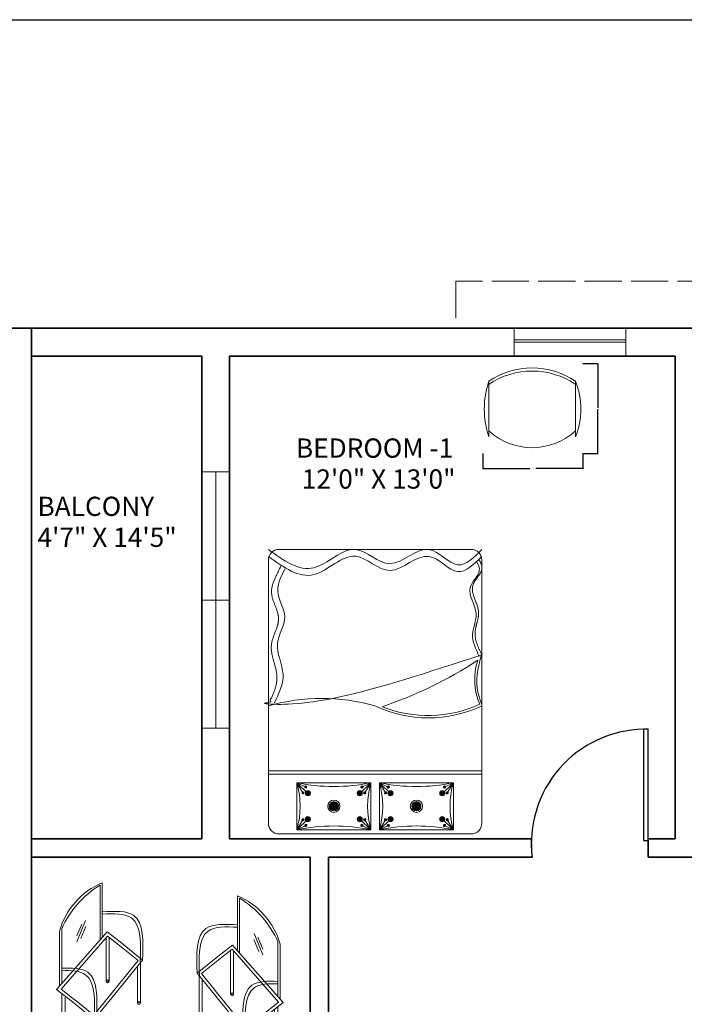
# Model space of a CAD drawing. Units: inches. Extents: x -61 to 1599, y -1316 to 257.
# Tile 201 of 204: x 998 to 1213, y -61 to 257. Entities that reach past the tile are written whole.
import ezdxf

# ---------------------------------------------------------------- set-up
doc = ezdxf.new("R2010")
doc.units = ezdxf.units.IN
doc.header["$MEASUREMENT"] = 0
doc.linetypes.add('ACAD_ISO02W100', pattern=[15, 12, -3])
for name, color, linetype, lineweight in [('A-ANNO-DIMS', 2, 'Continuous', 18), ('A-AREA-IDEN', 1, 'Continuous', 18), ('A-FLOR-OVHD', 203, 'ACAD_ISO02W100', 13), ('A-WALL-JAMB', 4, 'ACAD_ISO02W100', 25), ('DOORS', 2, 'Continuous', 25), ('FURNITURE', 83, 'Continuous', 18), ('WALLS', 4, 'Continuous', 35), ('WINDOWS', 220, 'Continuous', 18)]:
    doc.layers.add(name, color=color, linetype=linetype, lineweight=lineweight)
doc.layers.add('LT', color=8, linetype='Continuous')
doc.styles.get("Standard").update_dxf_attribs({"font": 'arial.ttf'})
doc.dimstyles.get("Standard").update_dxf_attribs({"dimtxt": 0.18, "dimasz": 0.18, "dimexe": 0.18, "dimexo": 0.0625, "dimgap": 0.09, "dimtad": 0, "dimtih": 1, "dimtoh": 1, "dimdec": 0, "dimzin": 0, "dimdsep": 46, "dimlunit": 3, "dimtxsty": 'Standard', "dimcen": 0.09, "dimadec": 0, "dimazin": 0, "dimtfac": 1, "dimtdec": 0, "dimtofl": 0, "dimtmove": 0, "dimatfit": 3, "dimfxl": 1, "dimtolj": 1, "dimtzin": 0, "dimarcsym": 0})

# ---------------------------------------------------------------- blocks, each defined once
blk = doc.blocks.new('DOOR-SWING-36')
blk.add_line((0, 0), (0, -5.4))
blk.add_lwpolyline([(0, 0), (0, 36), (-1.57, 36), (-1.57, 0)], close=True)
blk.add_arc((-0.74, -1.08), 37.09, 91.2913, 186.6905)
blk = doc.blocks.new('WIN-36IN')
for p, q in [((0, 4.5), (0, 9)), ((0, 9), (0, 0)), ((36, 9), (36, 0)), ((0, 5.26), (36, 5.26)), ((0, 4.5), (36, 4.5)), ((0, 4.5), (36, 4.5))]:
    blk.add_line(p, q)
blk = doc.blocks.new('WIN-83IN')
for p, q in [((0, 82.94), (9, 82.94)), ((0, 0), (9, 0))]:
    blk.add_line(p, q)
for points in [[(9, 82.94), (4.5, 82.94), (4.5, 41.47), (9, 41.47)], [(4.5, 41.47), (0, 41.47), (0, 0), (4.5, 0)]]:
    blk.add_lwpolyline(points, close=True)
blk = doc.blocks.new('BEDROOM-CHAIR')
for p, q in [((1.45, 3.47), (1.45, 21.47)), ((29.49, 3.47), (29.49, 21.47))]:
    blk.add_line(p, q)
for centre, radius, start, end in [((15.47, 0.83), 24.95, 55.8098, 124.1902), ((15.47, -0.17), 24.95, 55.8098, 124.1902), ((28.58, 12.47), 28.58, 161.6455, 198.3545), ((7.26, 12.47), 23.99, 337.9646, 22.0354), ((15.47, 20.69), 20.68, 227.332, 312.668)]:
    blk.add_arc(centre, radius, start, end)
blk = doc.blocks.new('LOUNGE-CHAIR')
for p, q in [((14.04, 40.33), (14.04, 58.08)), ((14.76, 41.14), (14.76, 58.89)), ((6.52, 39.78), (9.29, 46.65)), ((6.58, 41.68), (8.18, 45.54)), ((7.84, 40.87), (9.45, 44.74)), ((0, 24.35), (16.38, 42.98)), ((0.97, 25.45), (0.97, 43.2)), ((0.97, 25.45), (0.97, 43.2)), ((1.45, 24.49), (16.5, 41.61)), ((1.64, 26.22), (1.64, 43.97)), ((16.38, 42.98), (20.51, 39.74)), ((16.5, 41.61), (19.89, 38.96)), ((16.97, 42.52), (16.97, 42.52)), ((15.97, 27.05), (15.97, 41.01)), ((16.97, 27.05), (16.97, 41.25)), ((19.88, 38.97), (26.35, 33.72)), ((20.51, 39.74), (27.76, 33.87)), ((12.02, 16.03), (26.35, 33.72)), ((12.16, 14.63), (27.76, 33.87)), ((27.1, 20.02), (27.1, 33.05)), ((26.1, 20.02), (26.1, 31.82)), ((16.97, 27.05), (15.97, 27.05)), ((0, 24.35), (5.1, 20.35)), ((0.75, 23.69), (0.79, 23.74)), ((1.45, 24.49), (5.72, 21.14)), ((1.73, 7.53), (1.73, 23)), ((2.73, 7.53), (2.73, 22.21)), ((5.1, 20.35), (12.16, 14.63)), ((5.73, 21.13), (12.02, 16.03)), ((27.1, 20.02), (26.1, 20.02)), ((11.85, 0.5), (11.85, 14.88)), ((12.85, 0.5), (12.85, 15.48)), ((2.73, 7.53), (1.73, 7.53)), ((12.85, 0.5), (11.85, 0.5))]:
    blk.add_line(p, q)
for centre in [(16.47, 27.05), (26.6, 20.02), (2.23, 7.53), (12.35, 0.5)]:
    blk.add_circle(centre, 0.5)
for centre, radius, start, end in [((23.93, 36.92), 23.8, 112.6586, 164.6996), ((30.25, 31.33), 31.28, 121.203, 156.1552)]:
    blk.add_arc(centre, radius, start, end)
for points, knots in [([(14.76, 49.49), (18.73, 49.7), (28.38, 50.23), (27.99, 39.93), (27.76, 33.87)], [0, 0, 0, 0, 10.281855, 24.983674, 24.983674, 24.983674, 24.983674]), ([(14.76, 48.72), (18.48, 48.91), (27.65, 49.16), (27.27, 39.12), (27.05, 33.06), (27.04, 33.03), (27.04, 33.01), (27.04, 32.98)], [0.614676, 0.614676, 0.614676, 0.614676, 10.281855, 24.983674, 24.983674, 24.983674, 25.041855, 25.041855, 25.041855, 25.041855]), ([(1.64, 31.22), (4.99, 31.37), (13.47, 31.24), (13.11, 21.57), (12.88, 15.51)], [1.527723, 1.527723, 1.527723, 1.527723, 10.281855, 24.983674, 24.983674, 24.983674, 24.983674]), ([(1.64, 30.44), (4.72, 30.55), (12.75, 30.17), (12.39, 20.76), (12.17, 14.7), (12.16, 14.67), (12.16, 14.65), (12.16, 14.63)], [2.150702, 2.150702, 2.150702, 2.150702, 10.281855, 24.983674, 24.983674, 24.983674, 25.041855, 25.041855, 25.041855, 25.041855])]:
    blk.add_open_spline(points, degree=3, knots=knots)
blk = doc.blocks.new('*U15')
at = {"layer": 'LT'}
blk.add_line((0, 0.18), (0, -0.18), dxfattribs=at)
for centre, start, end in [((0.51, 0), 160.9983, 199.0017), ((-0.51, 0), 340.9983, 19.0017)]:
    blk.add_arc(centre, 0.539, start, end, dxfattribs=at)
blk = doc.blocks.new('*U16')
at = {"layer": 'LT', "transparency": 16777216}
for p, rotation in [((-66.65, -18.83), 96), ((-66.64, -18.76), 72), ((-66.63, -18.9), 120), ((-66.61, -18.69), 48.00000000000001), ((-66.58, -18.95), 144), ((-66.55, -18.65), 24), ((-66.51, -18.98), 168.0000000000001), ((-66.4, -18.65), 336.0000000000001), ((-66.37, -18.95), 216), ((-66.44, -18.98), 192), ((-66.34, -18.69), 312), ((-66.32, -18.9), 240), ((-66.31, -18.76), 288.0000000000001), ((-66.3, -18.83), 264)]:
    blk.add_blockref('*U15', p, dxfattribs=dict(at, rotation=rotation))
blk.add_blockref('*U15', (-66.48, -18.63), dxfattribs=at)
blk = doc.blocks.new('*U45')
at = {"layer": 'LT'}
blk.add_line((0, 0.18), (0, -0.18), dxfattribs=at)
for centre, start, end in [((0.51, 0), 160.9983, 199.0017), ((-0.51, 0), 340.9983, 19.0017)]:
    blk.add_arc(centre, 0.539, start, end, dxfattribs=at)
blk = doc.blocks.new('*U46')
at = {"layer": 'LT', "transparency": 16777216}
for p, rotation in [((-66.65, -18.83), 96), ((-66.64, -18.76), 72), ((-66.63, -18.9), 120), ((-66.61, -18.69), 48.00000000000001), ((-66.58, -18.95), 144), ((-66.55, -18.65), 24), ((-66.51, -18.98), 168.0000000000001), ((-66.4, -18.65), 336.0000000000001), ((-66.37, -18.95), 216), ((-66.44, -18.98), 192), ((-66.34, -18.69), 312), ((-66.32, -18.9), 240), ((-66.31, -18.76), 288.0000000000001), ((-66.3, -18.83), 264)]:
    blk.add_blockref('*U45', p, dxfattribs=dict(at, rotation=rotation))
blk.add_blockref('*U45', (-66.48, -18.63), dxfattribs=at)
blk = doc.blocks.new('*U9')
at = {"layer": 'LT'}
blk.add_line((0, 0.18), (0, -0.18), dxfattribs=at)
for centre, start, end in [((0.51, 0), 160.9983, 199.0017), ((-0.51, 0), 340.9983, 19.0017)]:
    blk.add_arc(centre, 0.539, start, end, dxfattribs=at)
blk = doc.blocks.new('*U10')
at = {"layer": 'LT', "transparency": 16777216}
for p, rotation in [((-66.65, -18.83), 96), ((-66.64, -18.76), 72), ((-66.63, -18.9), 120), ((-66.61, -18.69), 48.00000000000001), ((-66.58, -18.95), 144), ((-66.55, -18.65), 24), ((-66.51, -18.98), 168.0000000000001), ((-66.4, -18.65), 336.0000000000001), ((-66.37, -18.95), 216), ((-66.44, -18.98), 192), ((-66.34, -18.69), 312), ((-66.32, -18.9), 240), ((-66.31, -18.76), 288.0000000000001), ((-66.3, -18.83), 264)]:
    blk.add_blockref('*U9', p, dxfattribs=dict(at, rotation=rotation))
blk.add_blockref('*U9', (-66.48, -18.63), dxfattribs=at)
blk = doc.blocks.new('*U39')
at = {"layer": 'LT'}
blk.add_line((0, 0.18), (0, -0.18), dxfattribs=at)
for centre, start, end in [((0.51, 0), 160.9983, 199.0017), ((-0.51, 0), 340.9983, 19.0017)]:
    blk.add_arc(centre, 0.539, start, end, dxfattribs=at)
blk = doc.blocks.new('*U40')
at = {"layer": 'LT', "transparency": 16777216}
for p, rotation in [((-66.65, -18.83), 96), ((-66.64, -18.76), 72), ((-66.63, -18.9), 120), ((-66.61, -18.69), 48.00000000000001), ((-66.58, -18.95), 144), ((-66.55, -18.65), 24), ((-66.51, -18.98), 168.0000000000001), ((-66.4, -18.65), 336.0000000000001), ((-66.37, -18.95), 216), ((-66.44, -18.98), 192), ((-66.34, -18.69), 312), ((-66.32, -18.9), 240), ((-66.31, -18.76), 288.0000000000001), ((-66.3, -18.83), 264)]:
    blk.add_blockref('*U39', p, dxfattribs=dict(at, rotation=rotation))
blk.add_blockref('*U39', (-66.48, -18.63), dxfattribs=at)
blk = doc.blocks.new('*U17')
at = {"layer": 'LT'}
blk.add_line((0, 0.41), (0, -0.41), dxfattribs=at)
for centre, start, end in [((1.2, 0), 160.9983, 199.0017), ((-1.2, 0), 340.9983, 19.0017)]:
    blk.add_arc(centre, 1.27, start, end, dxfattribs=at)
blk = doc.blocks.new('*U18')
at = {"layer": 'LT', "transparency": 16777216}
for p, rotation in [((-156.74, -44.28), 96), ((-156.73, -44.11), 72), ((-156.69, -44.44), 120), ((-156.64, -43.96), 48.00000000000001), ((-156.58, -44.57), 144), ((-156.5, -43.86), 24), ((-156.42, -44.64), 168), ((-156.17, -43.86), 336.0000000000001), ((-156.25, -44.64), 192), ((-156.09, -44.57), 216), ((-156.03, -43.96), 312), ((-155.98, -44.44), 240), ((-155.94, -44.11), 288.0000000000001), ((-155.92, -44.28), 264)]:
    blk.add_blockref('*U17', p, dxfattribs=dict(at, rotation=rotation))
blk.add_blockref('*U17', (-156.33, -43.82), dxfattribs=at)
blk = doc.blocks.new('*U33')
at = {"layer": 'LT'}
blk.add_line((0, 0.41), (0, -0.41), dxfattribs=at)
for centre, start, end in [((1.2, 0), 160.9983, 199.0017), ((-1.2, 0), 340.9983, 19.0017)]:
    blk.add_arc(centre, 1.27, start, end, dxfattribs=at)
blk = doc.blocks.new('*U34')
at = {"layer": 'LT', "transparency": 16777216}
for p, rotation in [((-156.74, -44.28), 96), ((-156.73, -44.11), 72), ((-156.69, -44.44), 120), ((-156.64, -43.96), 48.00000000000001), ((-156.58, -44.57), 144), ((-156.5, -43.86), 24), ((-156.42, -44.64), 168), ((-156.17, -43.86), 336.0000000000001), ((-156.25, -44.64), 192), ((-156.09, -44.57), 216), ((-156.03, -43.96), 312), ((-155.98, -44.44), 240), ((-155.94, -44.11), 288.0000000000001), ((-155.92, -44.28), 264)]:
    blk.add_blockref('*U33', p, dxfattribs=dict(at, rotation=rotation))
blk.add_blockref('*U33', (-156.33, -43.82), dxfattribs=at)
blk = doc.blocks.new('*U11')
at = {"layer": 'LT'}
blk.add_line((0, 0.74), (0, -0.74), dxfattribs=at)
for centre, start, end in [((2.15, 0), 160.9983, 199.0017), ((-2.15, 0), 340.9983, 19.0017)]:
    blk.add_arc(centre, 2.27, start, end, dxfattribs=at)
blk = doc.blocks.new('*U12')
at = {"layer": 'LT', "transparency": 16777216}
for p, rotation in [((-280.98, -79.37), 96), ((-280.94, -79.07), 72), ((-280.88, -79.67), 120), ((-280.79, -78.8), 48.00000000000001), ((-280.68, -79.89), 144), ((-280.54, -78.62), 23.99999999999999), ((-280.4, -80.02), 168), ((-280.09, -80.02), 191.9999999999999), ((-279.94, -78.62), 336.0000000000001), ((-279.81, -79.89), 216), ((-279.69, -78.8), 312), ((-279.6, -79.67), 240), ((-279.54, -79.07), 288.0000000000001), ((-279.51, -79.37), 264)]:
    blk.add_blockref('*U11', p, dxfattribs=dict(at, rotation=rotation))
blk.add_blockref('*U11', (-280.24, -78.56), dxfattribs=at)
blk = doc.blocks.new('*U28')
at = {"layer": 'LT'}
blk.add_line((0, 0.41), (0, -0.41), dxfattribs=at)
for centre, start, end in [((1.2, 0), 160.9983, 199.0017), ((-1.2, 0), 340.9983, 19.0017)]:
    blk.add_arc(centre, 1.27, start, end, dxfattribs=at)
blk = doc.blocks.new('*U44')
at = {"layer": 'LT', "transparency": 16777216}
for p, rotation in [((-156.74, -44.28), 96), ((-156.73, -44.11), 72), ((-156.69, -44.44), 120), ((-156.64, -43.96), 48.00000000000001), ((-156.58, -44.57), 144), ((-156.5, -43.86), 24), ((-156.42, -44.64), 168), ((-156.17, -43.86), 336.0000000000001), ((-156.25, -44.64), 192), ((-156.09, -44.57), 216), ((-156.03, -43.96), 312), ((-155.98, -44.44), 240), ((-155.94, -44.11), 288.0000000000001), ((-155.92, -44.28), 264)]:
    blk.add_blockref('*U28', p, dxfattribs=dict(at, rotation=rotation))
blk.add_blockref('*U28', (-156.33, -43.82), dxfattribs=at)
blk = doc.blocks.new('*U13')
at = {"layer": 'LT'}
blk.add_line((0, 0.41), (0, -0.41), dxfattribs=at)
for centre, start, end in [((1.2, 0), 160.9983, 199.0017), ((-1.2, 0), 340.9983, 19.0017)]:
    blk.add_arc(centre, 1.27, start, end, dxfattribs=at)
blk = doc.blocks.new('*U14')
at = {"layer": 'LT', "transparency": 16777216}
for p, rotation in [((-156.74, -44.28), 96), ((-156.73, -44.11), 72), ((-156.69, -44.44), 120), ((-156.64, -43.96), 48.00000000000001), ((-156.58, -44.57), 144), ((-156.5, -43.86), 24), ((-156.42, -44.64), 168), ((-156.17, -43.86), 336.0000000000001), ((-156.25, -44.64), 192), ((-156.09, -44.57), 216), ((-156.03, -43.96), 312), ((-155.98, -44.44), 240), ((-155.94, -44.11), 288.0000000000001), ((-155.92, -44.28), 264)]:
    blk.add_blockref('*U13', p, dxfattribs=dict(at, rotation=rotation))
blk.add_blockref('*U13', (-156.33, -43.82), dxfattribs=at)
blk = doc.blocks.new('*U19')
at = {"layer": 'LT'}
blk.add_line((0, 0.18), (0, -0.18), dxfattribs=at)
for centre, start, end in [((0.51, 0), 160.9983, 199.0017), ((-0.51, 0), 340.9983, 19.0017)]:
    blk.add_arc(centre, 0.539, start, end, dxfattribs=at)
blk = doc.blocks.new('*U6')
at = {"layer": 'LT', "transparency": 16777216}
for p, rotation in [((-66.65, -18.83), 96), ((-66.64, -18.76), 72), ((-66.63, -18.9), 120), ((-66.61, -18.69), 48.00000000000001), ((-66.58, -18.95), 144), ((-66.55, -18.65), 24), ((-66.51, -18.98), 168.0000000000001), ((-66.4, -18.65), 336.0000000000001), ((-66.37, -18.95), 216), ((-66.44, -18.98), 192), ((-66.34, -18.69), 312), ((-66.32, -18.9), 240), ((-66.31, -18.76), 288.0000000000001), ((-66.3, -18.83), 264)]:
    blk.add_blockref('*U19', p, dxfattribs=dict(at, rotation=rotation))
blk.add_blockref('*U19', (-66.48, -18.63), dxfattribs=at)
blk = doc.blocks.new('*U35')
at = {"layer": 'LT'}
blk.add_line((0, 0.18), (0, -0.18), dxfattribs=at)
for centre, start, end in [((0.51, 0), 160.9983, 199.0017), ((-0.51, 0), 340.9983, 19.0017)]:
    blk.add_arc(centre, 0.539, start, end, dxfattribs=at)
blk = doc.blocks.new('*U36')
at = {"layer": 'LT', "transparency": 16777216}
for p, rotation in [((-66.65, -18.83), 96), ((-66.64, -18.76), 72), ((-66.63, -18.9), 120), ((-66.61, -18.69), 48.00000000000001), ((-66.58, -18.95), 144), ((-66.55, -18.65), 24), ((-66.51, -18.98), 168.0000000000001), ((-66.4, -18.65), 336.0000000000001), ((-66.37, -18.95), 216), ((-66.44, -18.98), 192), ((-66.34, -18.69), 312), ((-66.32, -18.9), 240), ((-66.31, -18.76), 288.0000000000001), ((-66.3, -18.83), 264)]:
    blk.add_blockref('*U35', p, dxfattribs=dict(at, rotation=rotation))
blk.add_blockref('*U35', (-66.48, -18.63), dxfattribs=at)
blk = doc.blocks.new('*U7')
at = {"layer": 'LT'}
blk.add_line((0, 0.18), (0, -0.18), dxfattribs=at)
for centre, start, end in [((0.51, 0), 160.9983, 199.0017), ((-0.51, 0), 340.9983, 19.0017)]:
    blk.add_arc(centre, 0.539, start, end, dxfattribs=at)
blk = doc.blocks.new('*U8')
at = {"layer": 'LT', "transparency": 16777216}
for p, rotation in [((-66.65, -18.83), 96), ((-66.64, -18.76), 72), ((-66.63, -18.9), 120), ((-66.61, -18.69), 48.00000000000001), ((-66.58, -18.95), 144), ((-66.55, -18.65), 24), ((-66.51, -18.98), 168.0000000000001), ((-66.4, -18.65), 336.0000000000001), ((-66.37, -18.95), 216), ((-66.44, -18.98), 192), ((-66.34, -18.69), 312), ((-66.32, -18.9), 240), ((-66.31, -18.76), 288.0000000000001), ((-66.3, -18.83), 264)]:
    blk.add_blockref('*U7', p, dxfattribs=dict(at, rotation=rotation))
blk.add_blockref('*U7', (-66.48, -18.63), dxfattribs=at)
blk = doc.blocks.new('*U37')
at = {"layer": 'LT'}
blk.add_line((0, 0.18), (0, -0.18), dxfattribs=at)
for centre, start, end in [((0.51, 0), 160.9983, 199.0017), ((-0.51, 0), 340.9983, 19.0017)]:
    blk.add_arc(centre, 0.539, start, end, dxfattribs=at)
blk = doc.blocks.new('*U38')
at = {"layer": 'LT', "transparency": 16777216}
for p, rotation in [((-66.65, -18.83), 96), ((-66.64, -18.76), 72), ((-66.63, -18.9), 120), ((-66.61, -18.69), 48.00000000000001), ((-66.58, -18.95), 144), ((-66.55, -18.65), 24), ((-66.51, -18.98), 168.0000000000001), ((-66.4, -18.65), 336.0000000000001), ((-66.37, -18.95), 216), ((-66.44, -18.98), 192), ((-66.34, -18.69), 312), ((-66.32, -18.9), 240), ((-66.31, -18.76), 288.0000000000001), ((-66.3, -18.83), 264)]:
    blk.add_blockref('*U37', p, dxfattribs=dict(at, rotation=rotation))
blk.add_blockref('*U37', (-66.48, -18.63), dxfattribs=at)
blk = doc.blocks.new('*U3')
at = {"layer": 'LT'}
blk.add_line((0, 0.18), (0, -0.18), dxfattribs=at)
for centre, start, end in [((0.51, 0), 160.9983, 199.0017), ((-0.51, 0), 340.9983, 19.0017)]:
    blk.add_arc(centre, 0.539, start, end, dxfattribs=at)
blk = doc.blocks.new('*U4')
at = {"layer": 'LT', "transparency": 16777216}
for p, rotation in [((-66.65, -18.83), 96), ((-66.64, -18.76), 72), ((-66.63, -18.9), 120), ((-66.61, -18.69), 48.00000000000001), ((-66.58, -18.95), 144), ((-66.55, -18.65), 24), ((-66.51, -18.98), 168.0000000000001), ((-66.4, -18.65), 336.0000000000001), ((-66.37, -18.95), 216), ((-66.44, -18.98), 192), ((-66.34, -18.69), 312), ((-66.32, -18.9), 240), ((-66.31, -18.76), 288.0000000000001), ((-66.3, -18.83), 264)]:
    blk.add_blockref('*U3', p, dxfattribs=dict(at, rotation=rotation))
blk.add_blockref('*U3', (-66.48, -18.63), dxfattribs=at)
blk = doc.blocks.new('*U20')
at = {"layer": 'LT'}
blk.add_line((0, 0.18), (0, -0.18), dxfattribs=at)
for centre, start, end in [((0.51, 0), 160.9983, 199.0017), ((-0.51, 0), 340.9983, 19.0017)]:
    blk.add_arc(centre, 0.539, start, end, dxfattribs=at)
blk = doc.blocks.new('*U21')
at = {"layer": 'LT', "transparency": 16777216}
for p, rotation in [((-66.65, -18.83), 96), ((-66.64, -18.76), 72), ((-66.63, -18.9), 120), ((-66.61, -18.69), 48.00000000000001), ((-66.58, -18.95), 144), ((-66.55, -18.65), 24), ((-66.51, -18.98), 168.0000000000001), ((-66.4, -18.65), 336.0000000000001), ((-66.37, -18.95), 216), ((-66.44, -18.98), 192), ((-66.34, -18.69), 312), ((-66.32, -18.9), 240), ((-66.31, -18.76), 288.0000000000001), ((-66.3, -18.83), 264)]:
    blk.add_blockref('*U20', p, dxfattribs=dict(at, rotation=rotation))
blk.add_blockref('*U20', (-66.48, -18.63), dxfattribs=at)
blk = doc.blocks.new('*U52')
at = {"layer": 'LT'}
blk.add_line((0, 0.18), (0, -0.18), dxfattribs=at)
for centre, start, end in [((0.51, 0), 160.9983, 199.0017), ((-0.51, 0), 340.9983, 19.0017)]:
    blk.add_arc(centre, 0.539, start, end, dxfattribs=at)
blk = doc.blocks.new('*U53')
at = {"layer": 'LT', "transparency": 16777216}
for p, rotation in [((-66.65, -18.83), 96), ((-66.64, -18.76), 72), ((-66.63, -18.9), 120), ((-66.61, -18.69), 48.00000000000001), ((-66.58, -18.95), 144), ((-66.55, -18.65), 24), ((-66.51, -18.98), 168.0000000000001), ((-66.4, -18.65), 336.0000000000001), ((-66.37, -18.95), 216), ((-66.44, -18.98), 192), ((-66.34, -18.69), 312), ((-66.32, -18.9), 240), ((-66.31, -18.76), 288.0000000000001), ((-66.3, -18.83), 264)]:
    blk.add_blockref('*U52', p, dxfattribs=dict(at, rotation=rotation))
blk.add_blockref('*U52', (-66.48, -18.63), dxfattribs=at)
blk = doc.blocks.new('*U29')
at = {"layer": 'LT'}
blk.add_line((0, 0.18), (0, -0.18), dxfattribs=at)
for centre, start, end in [((0.51, 0), 160.9983, 199.0017), ((-0.51, 0), 340.9983, 19.0017)]:
    blk.add_arc(centre, 0.539, start, end, dxfattribs=at)
blk = doc.blocks.new('*U30')
at = {"layer": 'LT', "transparency": 16777216}
for p, rotation in [((-66.65, -18.83), 96), ((-66.64, -18.76), 72), ((-66.63, -18.9), 120), ((-66.61, -18.69), 48.00000000000001), ((-66.58, -18.95), 144), ((-66.55, -18.65), 24), ((-66.51, -18.98), 168.0000000000001), ((-66.4, -18.65), 336.0000000000001), ((-66.37, -18.95), 216), ((-66.44, -18.98), 192), ((-66.34, -18.69), 312), ((-66.32, -18.9), 240), ((-66.31, -18.76), 288.0000000000001), ((-66.3, -18.83), 264)]:
    blk.add_blockref('*U29', p, dxfattribs=dict(at, rotation=rotation))
blk.add_blockref('*U29', (-66.48, -18.63), dxfattribs=at)
blk = doc.blocks.new('*U5')
at = {"layer": 'LT'}
blk.add_line((0, 0.41), (0, -0.41), dxfattribs=at)
for centre, start, end in [((1.2, 0), 160.9983, 199.0017), ((-1.2, 0), 340.9983, 19.0017)]:
    blk.add_arc(centre, 1.27, start, end, dxfattribs=at)
blk = doc.blocks.new('*U47')
at = {"layer": 'LT', "transparency": 16777216}
for p, rotation in [((-156.74, -44.28), 96), ((-156.73, -44.11), 72), ((-156.69, -44.44), 120), ((-156.64, -43.96), 48.00000000000001), ((-156.58, -44.57), 144), ((-156.5, -43.86), 24), ((-156.42, -44.64), 168), ((-156.17, -43.86), 336.0000000000001), ((-156.25, -44.64), 192), ((-156.09, -44.57), 216), ((-156.03, -43.96), 312), ((-155.98, -44.44), 240), ((-155.94, -44.11), 288.0000000000001), ((-155.92, -44.28), 264)]:
    blk.add_blockref('*U5', p, dxfattribs=dict(at, rotation=rotation))
blk.add_blockref('*U5', (-156.33, -43.82), dxfattribs=at)
blk = doc.blocks.new('*U22')
at = {"layer": 'LT'}
blk.add_line((0, 0.41), (0, -0.41), dxfattribs=at)
for centre, start, end in [((1.2, 0), 160.9983, 199.0017), ((-1.2, 0), 340.9983, 19.0017)]:
    blk.add_arc(centre, 1.27, start, end, dxfattribs=at)
blk = doc.blocks.new('*U23')
at = {"layer": 'LT', "transparency": 16777216}
for p, rotation in [((-156.74, -44.28), 96), ((-156.73, -44.11), 72), ((-156.69, -44.44), 120), ((-156.64, -43.96), 48.00000000000001), ((-156.58, -44.57), 144), ((-156.5, -43.86), 24), ((-156.42, -44.64), 168), ((-156.17, -43.86), 336.0000000000001), ((-156.25, -44.64), 192), ((-156.09, -44.57), 216), ((-156.03, -43.96), 312), ((-155.98, -44.44), 240), ((-155.94, -44.11), 288.0000000000001), ((-155.92, -44.28), 264)]:
    blk.add_blockref('*U22', p, dxfattribs=dict(at, rotation=rotation))
blk.add_blockref('*U22', (-156.33, -43.82), dxfattribs=at)
blk = doc.blocks.new('*U54')
at = {"layer": 'LT'}
blk.add_line((0, 0.74), (0, -0.74), dxfattribs=at)
for centre, start, end in [((2.15, 0), 160.9983, 199.0017), ((-2.15, 0), 340.9983, 19.0017)]:
    blk.add_arc(centre, 2.27, start, end, dxfattribs=at)
blk = doc.blocks.new('*U41')
at = {"layer": 'LT', "transparency": 16777216}
for p, rotation in [((-280.98, -79.37), 96), ((-280.94, -79.07), 72), ((-280.88, -79.67), 120), ((-280.79, -78.8), 48.00000000000001), ((-280.68, -79.89), 144), ((-280.54, -78.62), 23.99999999999999), ((-280.4, -80.02), 168), ((-280.09, -80.02), 191.9999999999999), ((-279.94, -78.62), 336.0000000000001), ((-279.81, -79.89), 216), ((-279.69, -78.8), 312), ((-279.6, -79.67), 240), ((-279.54, -79.07), 288.0000000000001), ((-279.51, -79.37), 264)]:
    blk.add_blockref('*U54', p, dxfattribs=dict(at, rotation=rotation))
blk.add_blockref('*U54', (-280.24, -78.56), dxfattribs=at)
blk = doc.blocks.new('*U42')
at = {"layer": 'LT'}
blk.add_line((0, 0.41), (0, -0.41), dxfattribs=at)
for centre, start, end in [((1.2, 0), 160.9983, 199.0017), ((-1.2, 0), 340.9983, 19.0017)]:
    blk.add_arc(centre, 1.27, start, end, dxfattribs=at)
blk = doc.blocks.new('*U43')
at = {"layer": 'LT', "transparency": 16777216}
for p, rotation in [((-156.74, -44.28), 96), ((-156.73, -44.11), 72), ((-156.69, -44.44), 120), ((-156.64, -43.96), 48.00000000000001), ((-156.58, -44.57), 144), ((-156.5, -43.86), 24), ((-156.42, -44.64), 168), ((-156.17, -43.86), 336.0000000000001), ((-156.25, -44.64), 192), ((-156.09, -44.57), 216), ((-156.03, -43.96), 312), ((-155.98, -44.44), 240), ((-155.94, -44.11), 288.0000000000001), ((-155.92, -44.28), 264)]:
    blk.add_blockref('*U42', p, dxfattribs=dict(at, rotation=rotation))
blk.add_blockref('*U42', (-156.33, -43.82), dxfattribs=at)
blk = doc.blocks.new('*U31')
at = {"layer": 'LT'}
blk.add_line((0, 0.41), (0, -0.41), dxfattribs=at)
for centre, start, end in [((1.2, 0), 160.9983, 199.0017), ((-1.2, 0), 340.9983, 19.0017)]:
    blk.add_arc(centre, 1.27, start, end, dxfattribs=at)
blk = doc.blocks.new('*U32')
at = {"layer": 'LT', "transparency": 16777216}
for p, rotation in [((-156.74, -44.28), 96), ((-156.73, -44.11), 72), ((-156.69, -44.44), 120), ((-156.64, -43.96), 48.00000000000001), ((-156.58, -44.57), 144), ((-156.5, -43.86), 24), ((-156.42, -44.64), 168), ((-156.17, -43.86), 336.0000000000001), ((-156.25, -44.64), 192), ((-156.09, -44.57), 216), ((-156.03, -43.96), 312), ((-155.98, -44.44), 240), ((-155.94, -44.11), 288.0000000000001), ((-155.92, -44.28), 264)]:
    blk.add_blockref('*U31', p, dxfattribs=dict(at, rotation=rotation))
blk.add_blockref('*U31', (-156.33, -43.82), dxfattribs=at)
blk = doc.blocks.new('*U48')
at = {"layer": 'LT'}
blk.add_line((0, 0.18), (0, -0.18), dxfattribs=at)
for centre, start, end in [((0.51, 0), 160.9983, 199.0017), ((-0.51, 0), 340.9983, 19.0017)]:
    blk.add_arc(centre, 0.539, start, end, dxfattribs=at)
blk = doc.blocks.new('*U49')
at = {"layer": 'LT', "transparency": 16777216}
for p, rotation in [((-66.65, -18.83), 96), ((-66.64, -18.76), 72), ((-66.63, -18.9), 120), ((-66.61, -18.69), 48.00000000000001), ((-66.58, -18.95), 144), ((-66.55, -18.65), 24), ((-66.51, -18.98), 168.0000000000001), ((-66.4, -18.65), 336.0000000000001), ((-66.37, -18.95), 216), ((-66.44, -18.98), 192), ((-66.34, -18.69), 312), ((-66.32, -18.9), 240), ((-66.31, -18.76), 288.0000000000001), ((-66.3, -18.83), 264)]:
    blk.add_blockref('*U48', p, dxfattribs=dict(at, rotation=rotation))
blk.add_blockref('*U48', (-66.48, -18.63), dxfattribs=at)
blk = doc.blocks.new('*U24')
at = {"layer": 'LT'}
blk.add_line((0, 0.18), (0, -0.18), dxfattribs=at)
for centre, start, end in [((0.51, 0), 160.9983, 199.0017), ((-0.51, 0), 340.9983, 19.0017)]:
    blk.add_arc(centre, 0.539, start, end, dxfattribs=at)
blk = doc.blocks.new('*U25')
at = {"layer": 'LT', "transparency": 16777216}
for p, rotation in [((-66.65, -18.83), 96), ((-66.64, -18.76), 72), ((-66.63, -18.9), 120), ((-66.61, -18.69), 48.00000000000001), ((-66.58, -18.95), 144), ((-66.55, -18.65), 24), ((-66.51, -18.98), 168.0000000000001), ((-66.4, -18.65), 336.0000000000001), ((-66.37, -18.95), 216), ((-66.44, -18.98), 192), ((-66.34, -18.69), 312), ((-66.32, -18.9), 240), ((-66.31, -18.76), 288.0000000000001), ((-66.3, -18.83), 264)]:
    blk.add_blockref('*U24', p, dxfattribs=dict(at, rotation=rotation))
blk.add_blockref('*U24', (-66.48, -18.63), dxfattribs=at)
blk = doc.blocks.new('*U50')
at = {"layer": 'LT'}
blk.add_line((0, 0.18), (0, -0.18), dxfattribs=at)
for centre, start, end in [((0.51, 0), 160.9983, 199.0017), ((-0.51, 0), 340.9983, 19.0017)]:
    blk.add_arc(centre, 0.539, start, end, dxfattribs=at)
blk = doc.blocks.new('*U51')
at = {"layer": 'LT', "transparency": 16777216}
for p, rotation in [((-66.65, -18.83), 96), ((-66.64, -18.76), 72), ((-66.63, -18.9), 120), ((-66.61, -18.69), 48.00000000000001), ((-66.58, -18.95), 144), ((-66.55, -18.65), 24), ((-66.51, -18.98), 168.0000000000001), ((-66.4, -18.65), 336.0000000000001), ((-66.37, -18.95), 216), ((-66.44, -18.98), 192), ((-66.34, -18.69), 312), ((-66.32, -18.9), 240), ((-66.31, -18.76), 288.0000000000001), ((-66.3, -18.83), 264)]:
    blk.add_blockref('*U50', p, dxfattribs=dict(at, rotation=rotation))
blk.add_blockref('*U50', (-66.48, -18.63), dxfattribs=at)
blk = doc.blocks.new('*U26')
at = {"layer": 'LT'}
blk.add_line((0, 0.18), (0, -0.18), dxfattribs=at)
for centre, start, end in [((0.51, 0), 160.9983, 199.0017), ((-0.51, 0), 340.9983, 19.0017)]:
    blk.add_arc(centre, 0.539, start, end, dxfattribs=at)
blk = doc.blocks.new('*U27')
at = {"layer": 'LT', "transparency": 16777216}
for p, rotation in [((-66.65, -18.83), 96), ((-66.64, -18.76), 72), ((-66.63, -18.9), 120), ((-66.61, -18.69), 48.00000000000001), ((-66.58, -18.95), 144), ((-66.55, -18.65), 24), ((-66.51, -18.98), 168.0000000000001), ((-66.4, -18.65), 336.0000000000001), ((-66.37, -18.95), 216), ((-66.44, -18.98), 192), ((-66.34, -18.69), 312), ((-66.32, -18.9), 240), ((-66.31, -18.76), 288.0000000000001), ((-66.3, -18.83), 264)]:
    blk.add_blockref('*U26', p, dxfattribs=dict(at, rotation=rotation))
blk.add_blockref('*U26', (-66.48, -18.63), dxfattribs=at)
blk = doc.blocks.new('BED-DOUBLE')
for p, q in [((1.27, 20.47), (70.26, 20.47)), ((1.27, 19.32), (70.26, 19.32)), ((10.47, 1.38), (10.47, 16.56)), ((34.39, 16.56), (10.47, 16.56)), ((10.47, 16.56), (13.35, 15.18)), ((10.47, 16.56), (14.04, 13.11)), ((10.47, 16.56), (12.45, 13.31)), ((34.39, 16.56), (30.82, 13.11)), ((34.39, 16.56), (31.51, 15.18)), ((34.39, 16.56), (32.4, 13.31)), ((37.15, 1.38), (37.15, 16.56)), ((61.06, 16.56), (37.15, 16.56)), ((37.15, 16.56), (40.03, 15.18)), ((37.15, 16.56), (40.71, 13.11)), ((37.15, 16.56), (39.13, 13.31)), ((61.06, 16.56), (57.5, 13.11)), ((61.06, 16.56), (58.18, 15.18)), ((61.06, 16.56), (59.08, 13.31)), ((12.45, 13.31), (12.45, 12.95)), ((13.35, 15.18), (13.35, 14.83)), ((14.05, 13.15), (14.05, 12.32)), ((30.81, 13.15), (30.81, 12.32)), ((31.51, 15.18), (31.51, 14.83)), ((32.4, 13.31), (32.4, 12.95)), ((39.13, 13.31), (39.13, 12.95)), ((40.03, 15.18), (40.03, 14.83)), ((40.73, 13.15), (40.73, 12.32)), ((57.48, 13.15), (57.48, 12.32)), ((58.18, 15.18), (58.18, 14.83)), ((59.08, 13.31), (59.08, 12.95)), ((22.43, 8.97), (22.43, 10.45)), ((49.11, 8.97), (49.11, 10.45)), ((10.47, 1.38), (14.04, 4.83)), ((10.47, 1.38), (12.45, 4.63)), ((12.45, 4.63), (12.45, 4.98)), ((14.05, 4.79), (14.05, 5.61)), ((30.81, 4.79), (30.81, 5.61)), ((34.39, 1.38), (30.82, 4.83)), ((32.4, 4.63), (32.4, 4.98)), ((34.39, 1.38), (32.4, 4.63)), ((37.15, 1.38), (40.71, 4.83)), ((37.15, 1.38), (39.13, 4.63)), ((39.13, 4.63), (39.13, 4.98)), ((40.73, 4.79), (40.73, 5.61)), ((57.48, 4.79), (57.48, 5.61)), ((61.06, 1.38), (57.5, 4.83)), ((59.08, 4.63), (59.08, 4.98)), ((61.06, 1.38), (59.08, 4.63)), ((10.47, 1.38), (13.35, 2.76)), ((13.35, 2.76), (13.35, 3.11)), ((31.51, 2.76), (31.51, 3.11)), ((34.39, 1.38), (31.51, 2.76)), ((34.39, 1.38), (34.39, 1.38)), ((37.15, 1.38), (40.03, 2.76)), ((40.03, 2.76), (40.03, 3.11)), ((58.18, 2.76), (58.18, 3.11)), ((61.06, 1.38), (58.18, 2.76)), ((61.06, 1.38), (61.06, 1.38))]:
    blk.add_line(p, q)
for points in [[(1.27, 88.54), (1.27, 3.45, 0.414214), (4.72, 0), (66.81, 0, 0.414214), (70.26, 3.45), (70.26, 88.54, 0.414214), (66.81, 91.99), (4.72, 91.99, 0.414214)], [(38.01, 41.13, 0.064396), (68.93, 56.18, 0.181766), (69.61, 41.92, -0.202767)], [(12.45, 13.31, 0.167358), (12.45, 12.95, 0.167358)], [(13.35, 15.18, 0.167358), (13.35, 14.83, 0.167358)], [(14.05, 13.15, 0.167358), (14.05, 12.32, 0.167358)], [(30.81, 12.32, 0.167358), (30.81, 13.15, 0.167358)], [(32.4, 12.95, 0.167358), (32.4, 13.31, 0.167358)], [(39.13, 13.31, 0.167358), (39.13, 12.95, 0.167358)], [(40.03, 15.18, 0.167358), (40.03, 14.83, 0.167358)], [(40.73, 13.15, 0.167358), (40.73, 12.32, 0.167358)], [(57.48, 12.32, 0.167358), (57.48, 13.15, 0.167358)], [(59.08, 12.95, 0.167358), (59.08, 13.31, 0.167358)], [(22.43, 8.97, 0.167358), (22.43, 10.45, 0.167358)], [(49.11, 8.97, 0.167358), (49.11, 10.45, 0.167358)], [(12.45, 4.98, 0.167358), (12.45, 4.63, 0.167358)], [(14.05, 5.61, 0.167358), (14.05, 4.79, 0.167358)], [(30.81, 4.79, 0.167358), (30.81, 5.61, 0.167358)], [(32.4, 4.63, 0.167358), (32.4, 4.98, 0.167358)], [(39.13, 4.98, 0.167358), (39.13, 4.63, 0.167358)], [(40.73, 5.61, 0.167358), (40.73, 4.79, 0.167358)], [(57.48, 4.79, 0.167358), (57.48, 5.61, 0.167358)], [(59.08, 4.63, 0.167358), (59.08, 4.98, 0.167358)], [(13.35, 3.11, 0.167358), (13.35, 2.76, 0.167358)], [(31.51, 2.76, 0.167358), (31.51, 3.11, 0.167358)], [(40.03, 3.11, 0.167358), (40.03, 2.76, 0.167358)], [(58.18, 2.76, 0.167358), (58.18, 3.11, 0.167358)]]:
    blk.add_lwpolyline(points, format="xyb", close=True)
blk.add_lwpolyline([(70.26, 41.39, -0.22309), (35.77, 41.39, 0.142156), (1.27, 41.39)], format="xyb")
for points in [[(34.39, 16.56), (34.39, 1.38), (10.47, 1.38), (10.47, 16.56), (34.39, 16.56), (34.39, 1.38), (10.47, 1.38)], [(61.06, 16.56), (61.06, 1.38), (37.15, 1.38)]]:
    blk.add_lwpolyline(points)
for centre, radius in [((12.45, 13.31), 0.351), ((13.35, 15.18), 0.351), ((14.05, 13.15), 0.825), ((30.81, 13.15), 0.825), ((31.51, 15.18), 0.351), ((32.4, 13.31), 0.351), ((39.13, 13.31), 0.351), ((40.03, 15.18), 0.351), ((40.73, 13.15), 0.825), ((57.48, 13.15), 0.825), ((58.18, 15.18), 0.351), ((59.08, 13.31), 0.351), ((22.43, 8.97), 1.98), ((22.43, 8.97), 1.48), ((49.11, 8.97), 1.98), ((49.11, 8.97), 1.48), ((12.45, 4.63), 0.351), ((14.05, 4.79), 0.825), ((30.81, 4.79), 0.825), ((32.4, 4.63), 0.351), ((39.13, 4.63), 0.351), ((40.73, 4.79), 0.825), ((57.48, 4.79), 0.825), ((59.08, 4.63), 0.351), ((13.35, 2.76), 0.351), ((31.51, 2.76), 0.351), ((40.03, 2.76), 0.351), ((58.18, 2.76), 0.351)]:
    blk.add_circle(centre, radius)
for centre, radius, start, end in [((-16, 8.97), 27.54, 344.0046, 15.9954), ((22.43, 74.54), 59.2, 258.3468, 281.6532), ((60.86, 8.97), 27.54, 164.0046, 195.9954), ((10.67, 8.97), 27.54, 344.0046, 15.9954), ((49.11, 74.54), 59.2, 258.3468, 281.6532), ((87.54, 8.97), 27.54, 164.0046, 195.9954), ((32.02, 15), 0.539, 160.9983, 199.0017), ((31, 15), 0.539, 340.9983, 19.0017), ((58.69, 15), 0.539, 160.9983, 199.0017), ((57.68, 15), 0.539, 340.9983, 19.0017), ((22.43, -56.6), 59.2, 78.3468, 101.6532), ((49.11, -56.6), 59.2, 78.3468, 101.6532)]:
    blk.add_arc(centre, radius, start, end)
for points, knots in [([(70.26, 91.99), (67.71, 89.38), (62.21, 83.76), (52.49, 96.72), (40.92, 82.74), (28.61, 96.74), (15.69, 81.53), (6.21, 88.41), (1.27, 91.99)], [0, 0, 0, 0, 9.176033, 19.753992, 33.150145, 45.209422, 59.881559, 75.764594, 75.764594, 75.764594, 75.764594]), ([(70.26, 89.76), (67.71, 87.16), (62.21, 81.54), (52.49, 94.5), (40.92, 80.52), (28.61, 94.52), (15.69, 79.31), (6.21, 86.19), (1.27, 89.76)], [0, 0, 0, 0, 9.176033, 19.753992, 33.150145, 45.209422, 59.881559, 75.764594, 75.764594, 75.764594, 75.764594]), ([(3.25, 42.44), (4.7, 45.45), (7.72, 51.72), (2.12, 61.25), (8.81, 70.52), (2.43, 77.93), (5.72, 83.91), (6.75, 86.04)], [0, 0, 0, 0, 8.27671, 17.241866, 24.903358, 33.244933, 38.427294, 38.427294, 38.427294, 38.427294]), ([(69.45, 57.36), (68.29, 59.79), (66.11, 64.34), (70.04, 71.91), (64.12, 79.11), (70.31, 84.4), (69.24, 87.09), (68.55, 88.05)], [0, 0, 0, 0, 6.649676, 12.451782, 19.973966, 25.324174, 28.349676, 28.349676, 28.349676, 28.349676])]:
    blk.add_open_spline(points, degree=3, knots=knots)
blk.add_open_spline([(5.01, 91.99), (4.99, 92.01), (4.96, 92.03), (4.94, 92.04)], degree=3)
for points, weights, knots in [([(70.26, 57.9), (59.86, 50.94), (48.6, 45.5), (36.68, 41.68), (36.46, 41.77), (36.25, 41.87), (36.03, 41.97), (24.6, 45.28), (12.69, 45.26), (1.27, 41.89), (2.72, 44.9), (5.74, 51.17), (0.14, 60.7), (6.83, 69.97), (0.11, 77.79), (4.35, 84.38), (5.4, 86.88)], [1, 0.993520320424, 0.993520320424, 1, 0.99997444972, 0.99997444972, 1, 0.973174868659, 0.973174868659, 1, 1, 1, 1, 1, 1, 1, 1], [0, 0, 0, 0, 0.279074, 0.279074, 0.279074, 0.296584, 0.296584, 0.296584, 0.865868, 0.865868, 0.865868, 9.142578, 18.107734, 25.769226, 34.110801, 40.441511, 40.441511, 40.441511, 40.441511]), ([(70.26, 41.83), (68.02, 47.03), (68.02, 52.7), (70.26, 57.9), (69.1, 60.33), (66.92, 64.87), (70.85, 72.44), (64.93, 79.65), (71.19, 84.99), (70.01, 87.73), (69.25, 88.74)], [1, 0.945466318698, 0.945466318698, 1, 1, 1, 1, 1, 1, 1, 1], [0, 0, 0, 0, 0.814571, 0.814571, 0.814571, 7.464247, 13.266353, 20.788537, 26.138745, 29.321895, 29.321895, 29.321895, 29.321895])]:
    blk.add_rational_spline(points, weights, degree=3, knots=knots)
for name, p in [('*U46', (78.93, 32.11)), ('*U40', (79.83, 33.99)), ('*U34', (170.39, 57.38)), ('*U21', (105.61, 32.11)), ('*U30', (106.5, 33.99)), ('*U23', (197.06, 57.38))]:
    blk.add_blockref(name, p)
at = {"extrusion": (0, 0, -1), "zscale": -1}
for name, p in [('*U14', (125.53, 57.38)), ('*U36', (34.97, 33.99)), ('*U38', (34.07, 32.11)), ('*U32', (98.85, 57.38)), ('*U25', (8.29, 33.99)), ('*U27', (7.39, 32.11))]:
    blk.add_blockref(name, p, dxfattribs=at)
at = {"rotation": 180}
for name, p in [('*U12', (-257.81, -70.33)), ('*U41', (-231.14, -70.33)), ('*U44', (-125.53, -39.45)), ('*U8', (-34.07, -14.18)), ('*U43', (-98.85, -39.45)), ('*U51', (-7.39, -14.18)), ('*U6', (-34.97, -16.05)), ('*U49', (-8.29, -16.05))]:
    blk.add_blockref(name, p, dxfattribs=at)
at = {"extrusion": (0, 0, -1), "zscale": -1, "rotation": 180}
for name, p in [('*U16', (-78.93, -14.18)), ('*U18', (-170.39, -39.45)), ('*U4', (-105.61, -14.18)), ('*U47', (-197.06, -39.45)), ('*U10', (-79.83, -16.05)), ('*U53', (-106.5, -16.05))]:
    blk.add_blockref(name, p, dxfattribs=at)
blk = doc.blocks.new('*D628')
at = {"layer": 'A-ANNO-DIMS', "color": 0, "lineweight": -2, "transparency": 16777216}
for p, q in [((1147.55, 117.19), (1147.55, 112.23)), ((1179.87, 117.19), (1179.87, 112.23)), ((1147.73, 112.41), (1162.76, 112.41)), ((1179.69, 112.41), (1164.66, 112.41))]:
    blk.add_line(p, q, dxfattribs=at)
at = {"layer": 'A-ANNO-DIMS', "color": 0, "transparency": 16777216}
for points in [[(1147.73, 112.44), (1147.73, 112.38), (1147.55, 112.41)], [(1179.69, 112.44), (1179.69, 112.38), (1179.87, 112.41)]]:
    blk.add_solid(points, dxfattribs=at)
at = {"layer": 'DEFPOINTS', "color": 0, "transparency": 16777216}
for p in [(1147.55, 117.25), (1179.87, 117.25), (1179.87, 112.41)]:
    blk.add_point(p, dxfattribs=at)
at = {"layer": 'A-ANNO-DIMS', "color": 0, "transparency": 16777216, "insert": (1163.71, 112.41), "char_height": 0.18, "attachment_point": 5}
blk.add_mtext('\\A1;CHAIR 32 TYP.', dxfattribs=at)
blk = doc.blocks.new('*D629')
at = {"layer": 'A-ANNO-DIMS', "color": 0, "lineweight": -2, "transparency": 16777216}
for p, q in [((1179.93, 146.29), (1184.89, 146.29)), ((1184.71, 146.11), (1184.71, 131.96)), ((1184.71, 117.43), (1184.71, 131.59)), ((1179.93, 117.25), (1184.89, 117.25))]:
    blk.add_line(p, q, dxfattribs=at)
at = {"layer": 'A-ANNO-DIMS', "color": 0, "transparency": 16777216}
for points in [[(1184.68, 146.11), (1184.74, 146.11), (1184.71, 146.29)], [(1184.68, 117.43), (1184.74, 117.43), (1184.71, 117.25)]]:
    blk.add_solid(points, dxfattribs=at)
at = {"layer": 'DEFPOINTS', "color": 0, "transparency": 16777216}
for p in [(1179.87, 146.29), (1184.71, 146.29), (1179.87, 117.25)]:
    blk.add_point(p, dxfattribs=at)
at = {"layer": 'A-ANNO-DIMS', "color": 0, "transparency": 16777216, "insert": (1184.71, 131.77), "char_height": 0.18, "attachment_point": 5}
blk.add_mtext('\\A1;29 TYP.', dxfattribs=at)
blk = doc.blocks.new('*D686')
at = {"layer": 'A-ANNO-DIMS', "color": 0, "lineweight": -2, "transparency": 16777216}
for p, q in [((14.7, 157.74), (14.7, 257.46)), ((14.88, 257.28), (768.35, 257.28)), ((1522.52, 257.28), (769.05, 257.28)), ((1522.7, 157.74), (1522.7, 257.46))]:
    blk.add_line(p, q, dxfattribs=at)
at = {"layer": 'A-ANNO-DIMS', "color": 0, "transparency": 16777216}
for points in [[(14.88, 257.31), (14.88, 257.25), (14.7, 257.28)], [(1522.52, 257.31), (1522.52, 257.25), (1522.7, 257.28)]]:
    blk.add_solid(points, dxfattribs=at)
at = {"layer": 'DEFPOINTS', "color": 0, "transparency": 16777216}
for p in [(1522.7, 257.28), (14.7, 157.68), (1522.7, 157.68)]:
    blk.add_point(p, dxfattribs=at)
at = {"layer": 'A-ANNO-DIMS', "color": 0, "transparency": 16777216, "insert": (768.7, 257.28), "char_height": 0.18, "attachment_point": 5}
blk.add_mtext('\\A1;1508', dxfattribs=at)

msp = doc.modelspace()

# ---------------------------------------------------------------- linework, layer by layer
at = {"layer": 'A-FLOR-OVHD'}
for p, q in [((1267.4807, 172.9695), (1138.8585, 172.9695)), ((1138.8585, 172.9695), (1138.8585, 157.6771))]:
    msp.add_line(p, q, dxfattribs=at)
at = {"layer": 'A-WALL-JAMB'}
for p, q in [((1163.4756, -13.3229), (1163.2611, -7.3229)), ((1201.0506, -13.3229), (1201.0506, -7.3229))]:
    msp.add_line(p, q, dxfattribs=at)
at = {"layer": 'WALLS'}
for p, q in [((1522.7028, 157.6771), (992.7028, 157.6771)), ((1001.7028, 157.6771), (1001.7028, -289.3229)), ((1001.7028, 148.6771), (1001.7028, -7.3229)), ((1001.7028, 148.6771), (1056.7028, 148.6771)), ((1056.7028, 148.6771), (1056.7028, -7.3229)), ((1065.7028, 148.6771), (1065.7028, -7.3229)), ((1065.7028, 148.6771), (1209.7028, 148.6771)), ((1209.7028, 148.6771), (1209.7028, -7.3229)), ((1001.7028, -7.3229), (1056.7028, -7.3229)), ((1065.7028, -7.3229), (1163.2611, -7.3229)), ((1201.0506, -7.3229), (1209.7028, -7.3229)), ((1001.7028, -13.3229), (1091.7028, -13.3229)), ((1001.7028, -169.3229), (1001.7028, -13.3229)), ((1091.7028, -169.3229), (1091.7028, -13.3229)), ((1097.7028, -13.3229), (1163.4756, -13.3229)), ((1097.7028, -169.3229), (1097.7028, -13.3229)), ((1201.0506, -13.3229), (1215.7028, -13.3229))]:
    msp.add_line(p, q, dxfattribs=at)

# ---------------------------------------------------------------- block references
at = {"layer": 'DOORS'}
msp.add_blockref('DOOR-SWING-36', (1201.0506, -7.9229), dxfattribs=at)
at = {"layer": 'FURNITURE'}
for name, p in [('BEDROOM-CHAIR', (1148.039, 119.079)), ('BED-DOUBLE', (1076.977, -5.797)), ('LOUNGE-CHAIR', (1009.776, -80.445))]:
    msp.add_blockref(name, p, dxfattribs=at)
at = {"layer": 'FURNITURE', "extrusion": (0, 0, -1), "zscale": -1}
msp.add_blockref('LOUNGE-CHAIR', (-1082.9843, -84.6679), dxfattribs=at)
at = {"layer": 'WINDOWS'}
for name, p in [('WIN-36IN', (1157.752, 148.677)), ('WIN-83IN', (1056.703, 28.365))]:
    msp.add_blockref(name, p, dxfattribs=at)

# ---------------------------------------------------------------- texts
at = {"layer": 'A-AREA-IDEN'}
for s, height, p in [('BEDROOM -1', 6.22364, (1087.1314, 115.8502)), (' 12\'0" X 13\'0"', 6.223643, (1087.1314, 105.8525)), ('BALCONY', 6.22364, (1003.5954, 97.019)), ('4\'7" X 14\'5"', 6.223643, (1003.5954, 87.0212))]:
    msp.add_text(s, height=height, dxfattribs=at).set_placement(p)

# ---------------------------------------------------------------- dimensions: what is measured, and where the dimension line sits
at = {"layer": 'A-ANNO-DIMS'}
dim = msp.add_linear_dim(base=(1522.7028, 257.2771), p1=(14.7028, 157.6771), p2=(1522.7028, 157.6771), dimstyle='Standard', override={"dimdec": 0, "dimlfac": 1, "dimrnd": 0, "dimzin": 0, "dimdsep": 46, "dimlunit": 2}, dxfattribs=at)
dim.commit()
dim.dimension.update_dxf_attribs({"geometry": '*D686', "text_midpoint": (768.7028, 257.2771)})
dim = msp.add_linear_dim(base=(1184.7146, 146.2939), p1=(1179.8676, 117.2543), p2=(1179.8676, 146.2939), angle=90, text='<> TYP.', dimstyle='Standard', override={"dimdec": 0, "dimlfac": 1, "dimrnd": 0, "dimzin": 0, "dimdsep": 46, "dimlunit": 2}, dxfattribs=at)
dim.commit()
dim.dimension.update_dxf_attribs({"geometry": '*D629', "text_midpoint": (1184.7146, 131.7741)})
dim = msp.add_linear_dim(base=(1179.8676, 112.4073), p1=(1147.5541, 117.2543), p2=(1179.8676, 117.2543), text='CHAIR <> TYP.', dimstyle='Standard', override={"dimdec": 0, "dimlfac": 1, "dimrnd": 0, "dimzin": 0, "dimdsep": 46, "dimlunit": 2}, dxfattribs=at)
dim.commit()
dim.dimension.update_dxf_attribs({"geometry": '*D628', "text_midpoint": (1163.7108, 112.4073)})

doc.saveas('drawing.dxf')
